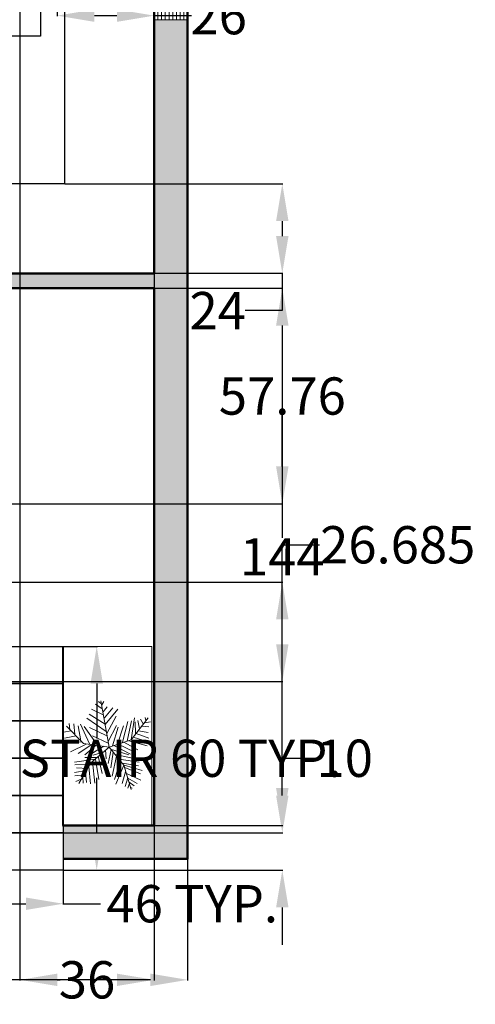
# Model space of a CAD drawing. Units: inches. Extents: x 133 to 758, y -29 to 543.
# Tile 4 of 7: x 590 to 712, y -29 to 235. Entities that reach past the tile are written whole.
import ezdxf

# ---------------------------------------------------------------- set-up
doc = ezdxf.new("R2010")
doc.units = ezdxf.units.IN
doc.header["$MEASUREMENT"] = 0
for name, color, linetype, lineweight in [('A-ANNO-DIMS', 2, 'Continuous', 18), ('A-FLOR-CASE', 32, 'Continuous', 25), ('A-FLOR-STRS', 7, 'Continuous', 25), ('A-WALL', 7, 'Continuous', 50), ('PLANT', 72, 'Continuous', 18), ('WINDOW', 151, 'Continuous', 18)]:
    doc.layers.add(name, color=color, linetype=linetype, lineweight=lineweight)
doc.layers.add('A-WALL-PATT', color=251, linetype='Continuous', lineweight=13, true_color=0x636466)
doc.styles.get("Standard").update_dxf_attribs({"font": 'arial.ttf'})
doc.dimstyles.get("Standard").update_dxf_attribs({"dimtxt": 10, "dimasz": 10, "dimexe": 0.18, "dimexo": 0.0625, "dimgap": 0.09, "dimtad": 0, "dimtih": 1, "dimtoh": 1, "dimdec": 0, "dimzin": 0, "dimdsep": 46, "dimlunit": 4, "dimtxsty": 'Standard', "dimcen": 0.09, "dimadec": 0, "dimazin": 0, "dimtfac": 1, "dimtdec": 0, "dimtofl": 0, "dimtmove": 0, "dimatfit": 3, "dimfxl": 1, "dimtolj": 1, "dimtzin": 0, "dimarcsym": 0})

# ---------------------------------------------------------------- blocks, each defined once
blk = doc.blocks.new('*U16')
for p, q in [((-221.9198, 1197.3052), (-433.5526, 1338.8594)), ((-258.7244, 1362.456), (-332.3336, 1421.4348)), ((0, 0), (-266.7, 1447.8)), ((-231.1146, 1315.2628), (-166.7002, 1421.4348)), ((-194.31, 1102.9442), (-65.4812, 1256.284)), ((-129.8956, 713.6638), (-626.7704, 1032.1544)), ((-185.1152, 1008.5578), (-553.1612, 1185.4942)), ((-148.3106, 914.1968), (118.5418, 1220.9018)), ((-129.8956, 701.8528), (265.7602, 1185.4942)), ((-74.7014, 418.7444), (219.7608, 961.39)), ((1121.4862, 925.9824), (1149.0706, 831.6214)), ((-800.1, 114.3), (-1333.5, 647.7)), ((-1234.059, 536.7274), (-1252.4486, 737.2604)), ((-1105.2302, 725.4494), (-1077.6458, 395.1732)), ((-976.4268, 666.4706), (-884.4026, 194.6402)), ((-902.8176, 713.6638), (-617.5756, 100.2538)), ((-369.1382, 53.086), (-783.1836, 642.874)), ((-93.091, 489.5342), (-700.3796, 902.3858)), ((-28.6766, 171.0436), (228.9556, 678.2816)), ((100.1268, 41.275), (284.1498, 619.2774)), ((256.5654, 88.4682), (449.7832, 666.4706)), ((412.9786, 147.447), (587.8068, 796.2392)), ((560.197, 182.8292), (698.2206, 819.8358)), ((685.8, 228.6), (1219.2, 914.4)), ((689.0258, 230.0224), (790.2448, 914.1968)), ((808.6344, 784.4282), (827.0494, 418.7444)), ((891.4384, 831.6214), (946.658, 572.1096)), ((983.4626, 867.0036), (1066.2666, 725.4494)), ((1029.462, 654.685), (1241.0948, 631.0884)), ((1112.2914, 760.8316), (1296.3144, 784.4282)), ((-1206.4492, 501.3198), (-1418.082, 465.9376)), ((-1031.621, 347.98), (-1399.667, 277.1902)), ((-617.5756, 607.4918), (-74.7014, 347.98)), ((-525.5514, 347.98), (-28.6766, 123.8504)), ((753.4148, 312.5978), (1222.6798, 159.2326)), ((845.439, 418.7444), (1241.0948, 277.1902)), ((919.0482, 501.3198), (1222.6798, 454.152)), ((-847.598, 159.2326), (-1326.0578, 135.636)), ((-718.7946, 88.4682), (-1215.644, -147.447)), ((-543.9664, 76.6572), (-967.2066, -206.4512)), ((0, 0), (-800.1, 114.3)), ((-405.9428, 53.086), (-764.794, -241.8334)), ((0, 0), (-571.5, -495.3)), ((-166.7002, 29.4894), (-543.9664, -206.4512)), ((0, 0), (685.8, 228.6)), ((0, 0), (457.2, -571.5)), ((164.5412, 41.275), (661.416, -218.2368)), ((284.1498, 88.4682), (781.0246, -147.447)), ((458.978, 147.447), (891.4384, -88.4682)), ((615.4166, 194.6402), (1185.8752, 41.275)), ((-166.7002, -147.447), (-507.1618, -253.619)), ((-341.5284, -289.0012), (-221.9198, -831.6214)), ((-240.3094, -218.2368), (-157.5054, -595.7062)), ((-120.7008, -88.4682), (-93.091, -371.5766)), ((63.3222, -76.6826), (-37.8714, -513.1308)), ((44.9326, -64.897), (615.4166, -241.8334)), ((127.7366, -159.258), (54.1274, -654.685)), ((228.9556, -289.0012), (90.932, -914.1968)), ((192.151, -230.0224), (817.8292, -371.5766)), ((-442.7474, -383.3876), (-1086.8406, -477.7486)), ((-617.5756, -548.5384), (-1077.6458, -560.324)), ((-571.5, -495.3), (-952.5, -1143)), ((-387.5278, -324.4088), (-764.794, -324.4088)), ((-635.9652, -607.5172), (-580.771, -1150.1374)), ((-525.5514, -465.963), (-451.9422, -1126.5408)), ((-433.5526, -383.3876), (-323.1134, -1020.3688)), ((357.759, -430.5554), (164.5412, -1020.3688)), ((458.978, -572.1096), (210.5406, -1161.923)), ((311.7596, -383.3876), (937.4378, -477.7486)), ((412.9786, -501.3452), (919.0482, -583.9206)), ((457.2, -571.5), (685.8, -1333.5)), ((468.1982, -572.1096), (1029.462, -737.2604)), ((-718.7946, -737.2604), (-1086.8406, -796.2392)), ((-783.1836, -867.029), (-1077.6458, -902.4112)), ((-681.9646, -666.496), (-1022.4262, -654.685)), ((-737.1842, -784.4536), (-709.5744, -1114.7298)), ((514.1976, -772.6426), (403.7838, -1138.3264)), ((486.5878, -642.8994), (983.4626, -843.4324)), ((541.8074, -831.6214), (992.6574, -1032.1544)), ((-875.2078, -1008.5832), (-1040.8412, -1079.3476)), ((-829.2084, -937.7934), (-810.7934, -1126.5408)), ((578.612, -961.39), (495.7826, -1232.7128)), ((578.612, -973.1756), (873.0488, -1138.3264)), ((624.6114, -1161.923), (587.8068, -1291.6916)), ((624.6114, -1102.9442), (781.0246, -1209.1162)), ((679.8056, -1268.095), (716.6102, -1291.6916))]:
    blk.add_line(p, q)
blk = doc.blocks.new('WIN-48IN')
for p, q in [((0, 8), (48, 8)), ((0, 7), (48, 7)), ((0, 6), (48, 6)), ((0, 5), (48, 5)), ((0, 4), (48, 4)), ((0, 3), (48, 3)), ((0, 2), (48, 2)), ((0, 1), (48, 1)), ((0, 0), (48, 0))]:
    blk.add_line(p, q)
blk.add_lwpolyline([(48, 9), (48, 0), (0, 0), (0, 9)], close=True)
blk = doc.blocks.new('PORCH-STAIR-6-TREAD')
blk.add_line((0, 60), (0, 0))
for points in [[(0, 60), (45.8, 60), (45.8, 50), (0, 50)], [(0, 50), (45.8, 50), (45.8, 40), (0, 40)], [(0, 40), (45.8, 40), (45.8, 30), (0, 30)], [(0, 30), (45.8, 30), (45.8, 20), (0, 20)], [(0, 20), (45.8, 20), (45.8, 10), (0, 10)], [(0, 10), (45.8, 10), (45.8, 0), (0, 0)]]:
    blk.add_lwpolyline(points)
blk = doc.blocks.new('PLANTER-24X48IN')
blk.add_lwpolyline([(0, 0), (24, 0), (24, 48), (0, 48)], close=True)
blk = doc.blocks.new('*D58')
at = {"layer": 'A-ANNO-DIMS', "color": 0, "lineweight": -2, "transparency": 16777216}
for p, q in [((601.41, 67.34), (610.53, 67.34)), ((610.35, 57.34), (610.35, 42.6)), ((610.35, 17.34), (610.35, 32.08)), ((601.41, 7.34), (610.53, 7.34))]:
    blk.add_line(p, q, dxfattribs=at)
at = {"layer": 'A-ANNO-DIMS', "color": 0, "transparency": 16777216}
for points in [[(608.68, 57.34), (612.02, 57.34), (610.35, 67.34)], [(608.68, 17.34), (612.02, 17.34), (610.35, 7.34)]]:
    blk.add_solid(points, dxfattribs=at)
at = {"layer": 'Defpoints', "color": 0, "transparency": 16777216}
for p in [(601.35, 67.34), (610.35, 67.34), (601.35, 7.34)]:
    blk.add_point(p, dxfattribs=at)
at = {"layer": 'A-ANNO-DIMS', "color": 0, "transparency": 16777216, "insert": (610.35, 37.34), "char_height": 10, "attachment_point": 5}
blk.add_mtext('\\A1;ENTRY STAIR 60 TYP.', dxfattribs=at)
blk = doc.blocks.new('*D59')
at = {"layer": 'A-ANNO-DIMS', "color": 0, "lineweight": -2, "transparency": 16777216}
for p, q in [((555.55, 7.27), (555.55, -1.84)), ((601.35, 7.27), (601.35, -1.84)), ((565.55, -1.66), (591.35, -1.66)), ((601.35, -1.66), (611.35, -1.66))]:
    blk.add_line(p, q, dxfattribs=at)
at = {"layer": 'A-ANNO-DIMS', "color": 0, "transparency": 16777216}
for points in [[(565.55, 0), (565.55, -3.33), (555.55, -1.66)], [(591.35, 0), (591.35, -3.33), (601.35, -1.66)]]:
    blk.add_solid(points, dxfattribs=at)
at = {"layer": 'Defpoints', "color": 0, "transparency": 16777216}
for p in [(555.55, 7.34), (601.35, 7.34), (601.35, -1.66)]:
    blk.add_point(p, dxfattribs=at)
at = {"layer": 'A-ANNO-DIMS', "color": 0, "transparency": 16777216, "insert": (635.98, -1.66), "char_height": 10, "attachment_point": 5}
blk.add_mtext('\\A1;46 TYP.', dxfattribs=at)
blk = doc.blocks.new('*D62')
at = {"layer": 'A-ANNO-DIMS', "color": 0, "lineweight": -2, "transparency": 16777216}
for p, q in [((599.69, 270.92), (595.07, 270.92)), ((595.25, 260.92), (595.25, 250.92)), ((599.69, 240.92), (595.07, 240.92)), ((595.25, 240.92), (595.25, 230.92)), ((595.25, 230.92), (585.25, 230.92))]:
    blk.add_line(p, q, dxfattribs=at)
at = {"layer": 'A-ANNO-DIMS', "color": 0, "transparency": 16777216}
for points in [[(593.58, 260.92), (596.92, 260.92), (595.25, 270.92)], [(593.58, 250.92), (596.92, 250.92), (595.25, 240.92)]]:
    blk.add_solid(points, dxfattribs=at)
at = {"layer": 'Defpoints', "color": 0, "transparency": 16777216}
for p in [(599.75, 270.92), (595.25, 240.92), (599.75, 240.92)]:
    blk.add_point(p, dxfattribs=at)
at = {"layer": 'A-ANNO-DIMS', "color": 0, "transparency": 16777216, "insert": (551.49, 230.92), "char_height": 10, "attachment_point": 5}
blk.add_mtext('\\A1;RANGE 30', dxfattribs=at)
blk = doc.blocks.new('*D63')
at = {"layer": 'A-ANNO-DIMS', "color": 0, "lineweight": -2, "transparency": 16777216}
for p, q in [((599.75, 240.86), (599.75, 236.24)), ((625.75, 240.86), (625.75, 236.24)), ((609.75, 236.42), (615.75, 236.42)), ((625.75, 236.42), (635.75, 236.42))]:
    blk.add_line(p, q, dxfattribs=at)
at = {"layer": 'A-ANNO-DIMS', "color": 0, "transparency": 16777216}
for points in [[(609.75, 238.09), (609.75, 234.75), (599.75, 236.42)], [(615.75, 238.09), (615.75, 234.75), (625.75, 236.42)]]:
    blk.add_solid(points, dxfattribs=at)
at = {"layer": 'Defpoints', "color": 0, "transparency": 16777216}
for p in [(599.75, 240.92), (625.75, 240.92), (625.75, 236.42)]:
    blk.add_point(p, dxfattribs=at)
at = {"layer": 'A-ANNO-DIMS', "color": 0, "transparency": 16777216, "insert": (643.08, 236.42), "char_height": 10, "attachment_point": 5}
blk.add_mtext('\\A1;26', dxfattribs=at)
blk = doc.blocks.new('*D72')
at = {"layer": 'A-ANNO-DIMS', "color": 0, "lineweight": -2, "transparency": 16777216}
for p, q in [((256.75, 10.27), (256.75, -22.24)), ((634.75, 10.27), (634.75, -22.24)), ((266.75, -22.06), (434.61, -22.06)), ((624.75, -22.06), (456.89, -22.06))]:
    blk.add_line(p, q, dxfattribs=at)
at = {"layer": 'A-ANNO-DIMS', "color": 0, "transparency": 16777216}
for points in [[(266.75, -20.4), (266.75, -23.73), (256.75, -22.06)], [(624.75, -20.4), (624.75, -23.73), (634.75, -22.06)]]:
    blk.add_solid(points, dxfattribs=at)
at = {"layer": 'Defpoints', "color": 0, "transparency": 16777216}
for p in [(256.75, 10.34), (634.75, 10.34), (634.75, -22.06)]:
    blk.add_point(p, dxfattribs=at)
at = {"layer": 'A-ANNO-DIMS', "color": 0, "transparency": 16777216, "insert": (445.75, -22.06), "char_height": 10, "attachment_point": 5}
blk.add_mtext('\\A1;378', dxfattribs=at)
blk = doc.blocks.new('*D81')
at = {"layer": 'A-ANNO-DIMS', "color": 0, "lineweight": -2, "transparency": 16777216}
for p, q in [((589.75, 499.27), (589.75, -22.24)), ((625.75, 499.27), (625.75, -22.24)), ((599.75, -22.06), (600.5, -22.06)), ((615.75, -22.06), (615, -22.06))]:
    blk.add_line(p, q, dxfattribs=at)
at = {"layer": 'A-ANNO-DIMS', "color": 0, "transparency": 16777216}
for points in [[(599.75, -20.4), (599.75, -23.73), (589.75, -22.06)], [(615.75, -20.4), (615.75, -23.73), (625.75, -22.06)]]:
    blk.add_solid(points, dxfattribs=at)
at = {"layer": 'Defpoints', "color": 0, "transparency": 16777216}
for p in [(589.75, 499.34), (625.75, 499.34), (625.75, -22.06)]:
    blk.add_point(p, dxfattribs=at)
at = {"layer": 'A-ANNO-DIMS', "color": 0, "transparency": 16777216, "insert": (607.75, -22.06), "char_height": 10, "attachment_point": 5}
blk.add_mtext('\\A1;36', dxfattribs=at)
blk = doc.blocks.new('*D86')
at = {"layer": 'A-ANNO-DIMS', "color": 0, "lineweight": -2, "transparency": 16777216}
for p, q in [((601.81, 191.34), (660.33, 191.34)), ((660.15, 181.34), (660.15, 177.34)), ((625.81, 167.34), (660.33, 167.34)), ((660.15, 167.34), (660.15, 157.34)), ((660.15, 157.34), (650.15, 157.34))]:
    blk.add_line(p, q, dxfattribs=at)
at = {"layer": 'A-ANNO-DIMS', "color": 0, "transparency": 16777216}
for points in [[(658.48, 181.34), (661.82, 181.34), (660.15, 191.34)], [(658.48, 177.34), (661.82, 177.34), (660.15, 167.34)]]:
    blk.add_solid(points, dxfattribs=at)
at = {"layer": 'Defpoints', "color": 0, "transparency": 16777216}
for p in [(601.75, 191.34), (625.75, 167.34), (660.15, 167.34)]:
    blk.add_point(p, dxfattribs=at)
at = {"layer": 'A-ANNO-DIMS', "color": 0, "transparency": 16777216, "insert": (642.83, 157.34), "char_height": 10, "attachment_point": 5}
blk.add_mtext('\\A1;24', dxfattribs=at)
blk = doc.blocks.new('*D88')
at = {"layer": 'A-ANNO-DIMS', "color": 0, "lineweight": -2, "transparency": 16777216}
for p, q in [((625.81, 163.34), (660.33, 163.34)), ((660.15, 153.34), (660.15, 96.45)), ((660.15, 29.34), (660.15, 86.23)), ((625.81, 19.34), (660.33, 19.34))]:
    blk.add_line(p, q, dxfattribs=at)
at = {"layer": 'A-ANNO-DIMS', "color": 0, "transparency": 16777216}
for points in [[(658.48, 153.34), (661.82, 153.34), (660.15, 163.34)], [(658.48, 29.34), (661.82, 29.34), (660.15, 19.34)]]:
    blk.add_solid(points, dxfattribs=at)
at = {"layer": 'Defpoints', "color": 0, "transparency": 16777216}
for p in [(625.75, 163.34), (660.15, 163.34), (625.75, 19.34)]:
    blk.add_point(p, dxfattribs=at)
at = {"layer": 'A-ANNO-DIMS', "color": 0, "transparency": 16777216, "insert": (660.15, 91.34), "char_height": 10, "attachment_point": 5}
blk.add_mtext('\\A1;144', dxfattribs=at)
blk = doc.blocks.new('*D93')
at = {"layer": 'A-ANNO-DIMS', "color": 0, "lineweight": -2, "transparency": 16777216}
for p, q in [((477.81, 163.34), (660.33, 163.34)), ((660.15, 153.34), (660.15, 139.65)), ((660.15, 115.57), (660.15, 129.26)), ((475.03, 105.57), (660.33, 105.57))]:
    blk.add_line(p, q, dxfattribs=at)
at = {"layer": 'A-ANNO-DIMS', "color": 0, "transparency": 16777216}
for points in [[(658.48, 153.34), (661.82, 153.34), (660.15, 163.34)], [(658.48, 115.57), (661.82, 115.57), (660.15, 105.57)]]:
    blk.add_solid(points, dxfattribs=at)
at = {"layer": 'Defpoints', "color": 0, "transparency": 16777216}
for p in [(477.75, 163.34), (660.15, 163.34), (474.97, 105.57)]:
    blk.add_point(p, dxfattribs=at)
at = {"layer": 'A-ANNO-DIMS', "color": 0, "transparency": 16777216, "insert": (660.15, 134.45), "char_height": 10, "attachment_point": 5}
blk.add_mtext('\\A1;57.76', dxfattribs=at)
blk = doc.blocks.new('*D94')
at = {"layer": 'A-ANNO-DIMS', "color": 0, "lineweight": -2, "transparency": 16777216}
for p, q in [((660.15, 84.57), (660.15, 94.57)), ((660.15, 94.57), (670.15, 94.57)), ((475.03, 84.57), (660.33, 84.57)), ((660.15, 67.89), (660.15, 74.57)), ((474.23, 57.89), (660.33, 57.89))]:
    blk.add_line(p, q, dxfattribs=at)
at = {"layer": 'A-ANNO-DIMS', "color": 0, "transparency": 16777216}
for points in [[(658.48, 74.57), (661.82, 74.57), (660.15, 84.57)], [(658.48, 67.89), (661.82, 67.89), (660.15, 57.89)]]:
    blk.add_solid(points, dxfattribs=at)
at = {"layer": 'Defpoints', "color": 0, "transparency": 16777216}
for p in [(474.97, 84.57), (660.15, 84.57), (474.17, 57.89)]:
    blk.add_point(p, dxfattribs=at)
at = {"layer": 'A-ANNO-DIMS', "color": 0, "transparency": 16777216, "insert": (691.12, 94.57), "char_height": 10, "attachment_point": 5}
blk.add_mtext('\\A1;26.685', dxfattribs=at)
blk = doc.blocks.new('*D95')
at = {"layer": 'A-ANNO-DIMS', "color": 0, "lineweight": -2, "transparency": 16777216}
for p, q in [((660.15, 27.34), (660.15, 37.34)), ((660.15, 37.34), (670.15, 37.34)), ((601.41, 17.34), (660.33, 17.34)), ((601.41, 7.34), (660.33, 7.34)), ((660.15, -2.66), (660.15, -12.66))]:
    blk.add_line(p, q, dxfattribs=at)
at = {"layer": 'A-ANNO-DIMS', "color": 0, "transparency": 16777216}
for points in [[(658.48, 27.34), (661.82, 27.34), (660.15, 17.34)], [(658.48, -2.66), (661.82, -2.66), (660.15, 7.34)]]:
    blk.add_solid(points, dxfattribs=at)
at = {"layer": 'Defpoints', "color": 0, "transparency": 16777216}
for p in [(601.35, 17.34), (660.15, 17.34), (601.35, 7.34)]:
    blk.add_point(p, dxfattribs=at)
at = {"layer": 'A-ANNO-DIMS', "color": 0, "transparency": 16777216, "insert": (676.91, 37.34), "char_height": 10, "attachment_point": 5}
blk.add_mtext('\\A1;10', dxfattribs=at)

msp = doc.modelspace()

# ---------------------------------------------------------------- hatches: boundary and pattern name
at = {"layer": 'A-WALL-PATT'}
h = msp.add_hatch(color=256, dxfattribs=at)
h.dxf.hatch_style = 1
h.paths.add_polyline_path([(634.7501, 235.336), (625.7501, 235.336), (625.7501, 167.336), (529.7501, 167.336), (529.7501, 211.336), (525.7501, 211.336), (525.7501, 167.336), (511.7501, 167.336), (511.7501, 163.336), (625.7501, 163.336), (625.7501, 19.336), (625.1804, 19.336), (601.3503, 19.336), (601.3503, 17.336), (601.3503, 10.336), (634.7501, 10.336)])

# ---------------------------------------------------------------- linework, layer by layer
at = {"layer": 'A-FLOR-CASE'}
for p, q in [((601.7501, 351.336), (601.7501, 191.336)), ((601.7501, 191.336), (529.7501, 191.336))]:
    msp.add_line(p, q, dxfattribs=at)
at = {"layer": 'A-WALL'}
for p, q in [((625.7501, 351.336), (625.7501, 167.336)), ((625.7501, 167.336), (529.7501, 167.336)), ((625.7501, 163.336), (511.7501, 163.336)), ((625.7501, 163.336), (625.7501, 19.336)), ((625.7501, 19.336), (601.1804, 19.336))]:
    msp.add_line(p, q, dxfattribs=at)
msp.add_lwpolyline([(505.7501, 10.336), (256.7501, 10.336), (256.7501, 508.336), (634.7501, 508.336), (634.7501, 10.336), (601.3503, 10.336)], dxfattribs=at)

# ---------------------------------------------------------------- block references
at = {"layer": 'A-FLOR-STRS'}
msp.add_blockref('PORCH-STAIR-6-TREAD', (555.55, 7.336), dxfattribs=at)
at = {"layer": 'PLANT'}
msp.add_blockref('PLANTER-24X48IN', (601.1803, 19.336), dxfattribs=at)
at = {"layer": 'PLANT', "xscale": 0.0085716703265903, "yscale": 0.0085716703265903, "zscale": 0.0085716703265903}
msp.add_blockref('*U16', (613.7045, 40.3482), dxfattribs=at)
at = {"layer": 'WINDOW', "rotation": 270.0000000000001}
msp.add_blockref('WIN-48IN', (625.7501, 283.3362), dxfattribs=at)

# ---------------------------------------------------------------- dimensions: what is measured, and where the dimension line sits
at = {"layer": 'A-ANNO-DIMS'}
for base, p1, p2, picture, middle in [((625.7501, -22.064), (589.7501, 499.336), (625.7501, 499.336), '*D81', (607.7501, -22.064)), ((625.7501, 236.4203), (599.7501, 240.9203), (625.7501, 240.9203), '*D63', (643.0843, 236.4203)), ((634.7501, -22.064), (256.7501, 10.336), (634.7501, 10.336), '*D72', (445.7501, -22.064))]:
    dim = msp.add_linear_dim(base=base, p1=p1, p2=p2, dimstyle='Standard', override={"dimdec": 0, "dimlfac": 1, "dimrnd": 0, "dimzin": 0, "dimdsep": 46, "dimlunit": 2}, dxfattribs=at)
    dim.commit()
    dim.dimension.update_dxf_attribs({"geometry": picture, "text_midpoint": middle})
for base, p1, p2, angle, text, picture, middle in [((595.2501, 240.9203), (599.7501, 270.9203), (599.7501, 240.9203), 270, 'RANGE <>', '*D62', (551.4937, 230.9203)), ((610.3503, 67.336), (601.3503, 7.336), (601.3503, 67.336), 90, 'ENTRY STAIR <> TYP.', '*D58', (610.3503, 37.336))]:
    dim = msp.add_linear_dim(base=base, p1=p1, p2=p2, angle=angle, text=text, dimstyle='Standard', override={"dimdec": 0, "dimlfac": 1, "dimrnd": 0, "dimzin": 0, "dimdsep": 46, "dimlunit": 2}, dxfattribs=at)
    dim.commit()
    dim.dimension.update_dxf_attribs({"geometry": picture, "text_midpoint": middle})
for base, p1, p2, override, picture, middle in [((660.1501, 167.336), (601.7501, 191.336), (625.7501, 167.336), {"dimdec": 0, "dimlfac": 1, "dimrnd": 0, "dimzin": 0, "dimdsep": 46, "dimlunit": 2}, '*D86', (642.833, 157.336)), ((660.1501, 163.336), (474.9703, 105.5711), (477.7501, 163.336), {"dimdec": 2, "dimlfac": 1, "dimrnd": 0, "dimzin": 0, "dimdsep": 46, "dimlunit": 2}, '*D93', (660.1501, 134.4536)), ((660.1501, 163.336), (625.7501, 19.336), (625.7501, 163.336), {"dimdec": 0, "dimlfac": 1, "dimrnd": 0, "dimzin": 0, "dimdsep": 46, "dimlunit": 2}, '*D88', (660.1501, 91.336)), ((660.1501, 84.5711), (474.1676, 57.886), (474.9703, 84.5711), {"dimdec": 3, "dimlfac": 1, "dimrnd": 0, "dimzin": 0, "dimdsep": 46, "dimlunit": 2}, '*D94', (691.1201, 94.5711)), ((660.1501, 17.336), (601.3503, 7.336), (601.3503, 17.336), {"dimdec": 0, "dimlfac": 1, "dimrnd": 0, "dimzin": 0, "dimdsep": 46, "dimlunit": 2}, '*D95', (676.9147, 37.336))]:
    dim = msp.add_linear_dim(base=base, p1=p1, p2=p2, angle=90, dimstyle='Standard', override=override, dxfattribs=at)
    dim.commit()
    dim.dimension.update_dxf_attribs({"geometry": picture, "text_midpoint": middle})
dim = msp.add_linear_dim(base=(601.3503, -1.664), p1=(555.5502, 7.336), p2=(601.3503, 7.336), text='<> TYP.', dimstyle='Standard', override={"dimdec": 0, "dimlfac": 1, "dimrnd": 0, "dimzin": 0, "dimdsep": 46, "dimlunit": 2}, dxfattribs=at)
dim.commit()
dim.dimension.update_dxf_attribs({"geometry": '*D59', "text_midpoint": (635.9799, -1.664)})

doc.saveas('drawing.dxf')
